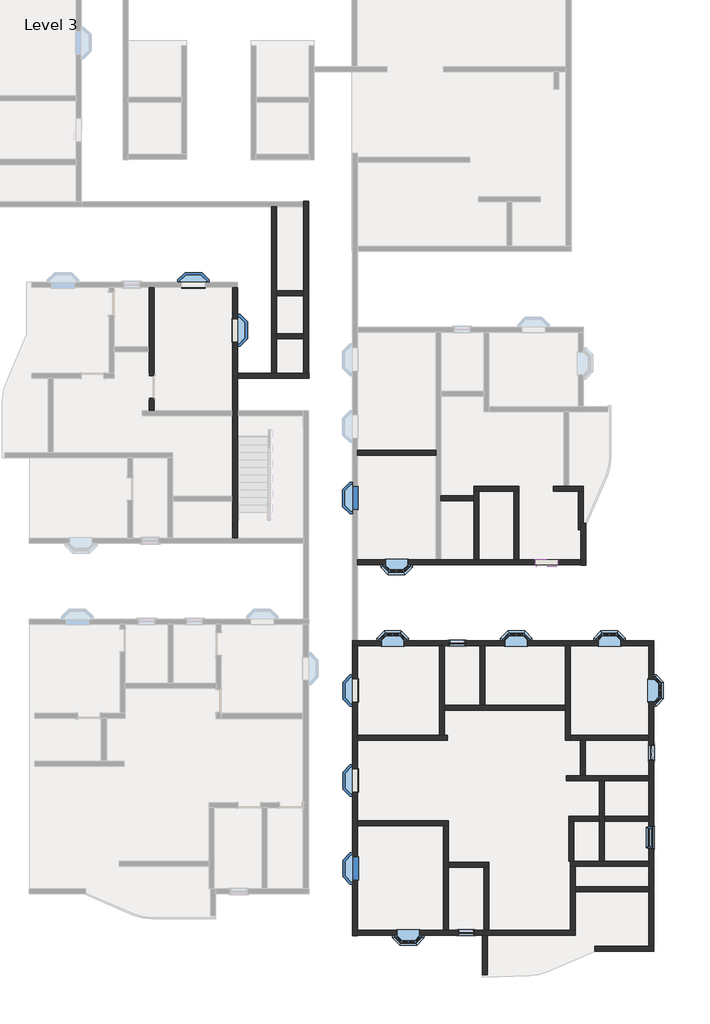
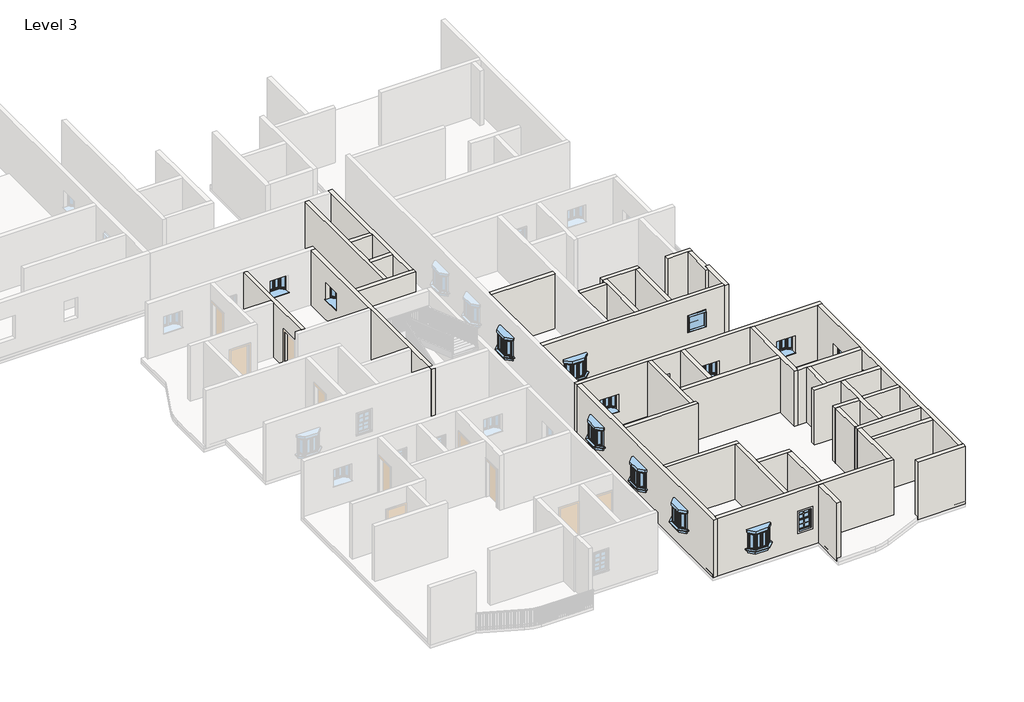
# One storey, part 2 of 14: 40 walls, 17 windows.
# Revit data of these elements (continued)
# Element 46 (IfcWindow, "910x910mm") (continued)
#   Materials on its faces: "Window Frame", "Glass"
# Element 47 (IfcWindow, "910x910mm")
#   Mark = "136"
#   Phase Created = New Construction
#   Materials on its faces: "Window Frame", "Glass"
# Element 48 (IfcWindow, "910x910mm")
#   Mark = "137"
#   Phase Created = New Construction
#   Materials on its faces: "Window Frame", "Glass"
# Element 49 (IfcWindow, "910x910mm")
#   Mark = "138"
#   Phase Created = New Construction
#   Materials on its faces: "Window Frame", "Glass"
# Element 50 (IfcWindow, "910x910mm")
#   Mark = "139"
#   Phase Created = New Construction
#   Materials on its faces: "Window Frame", "Glass"
# Element 51 (IfcWindow, "910x910mm")
#   Mark = "140"
#   Phase Created = New Construction
#   Materials on its faces: "Window Frame", "Glass"
# Element 52 (IfcWindow, "910x910mm")
#   Mark = "141"
#   Phase Created = New Construction
#   Materials on its faces: "Window Frame", "Glass"
# Element 53 (IfcWindow, "Window-Double-Hung : 26\" x 42\"")
#   Mark = "164"
#   Window Inset = 0' - 0"
#   Interior Wall Closure = 0' - 1 1/2"
#   Frame Extension = 0' - 1 1/4"
#   Exterior Wall Closure = 0' - 0 1/2"
#   Interior Trim Visibility = yes
#   Indicator Visibility = yes
#   Exterior Trim Visibility = yes
#   Phase Created = New Construction
#   Materials on its faces: "Wood - Stained", "Glass", "Clad - White"
# Element 54 (IfcWindow, "Window-Double-Hung : 26\" x 42\"")
#   Mark = "165"
#   Window Inset = 0' - 0"
#   Interior Wall Closure = 0' - 1 1/2"
#   Frame Extension = 0' - 1 1/4"
#   Exterior Wall Closure = 0' - 0 1/2"
#   Interior Trim Visibility = yes
#   Indicator Visibility = yes
#   Exterior Trim Visibility = yes
#   Phase Created = New Construction
#   Materials on its faces: "Wood - Stained", "Glass", "Clad - White"
# Element 55 (IfcWindow, "Window-Double-Hung : 26\" x 42\"")
#   Mark = "166"
#   Window Inset = 0' - 0"
#   Interior Wall Closure = 0' - 1 1/2"
#   Frame Extension = 0' - 1 1/4"
#   Exterior Wall Closure = 0' - 0 1/2"
#   Interior Trim Visibility = yes
#   Indicator Visibility = yes
#   Exterior Trim Visibility = yes
#   Phase Created = New Construction
#   Materials on its faces: "Wood - Stained", "Glass", "Clad - White"
# Element 56 (IfcWindow, "Windows_Sgl_w-Glazing_Bars : 910x910mm")
#   Mark = "154"
#   Phase Created = New Construction
#   Materials on its faces: "Window Frame", "Glass"
# Element 57 (IfcWindow, "Windows_Sgl_w-Glazing_Bars : 910x910mm")
#   Mark = "153"
#   Phase Created = New Construction
#   Materials on its faces: "Window Frame", "Glass"
# Materials
#   "Window Frame": colour RGB 249 249 249, transparency 0
#   "Glass": class "Glass", colour RGB 0 128 192, transparency 0.75, Description = "Soda Lime Glass", Cost = 0
#   "Wood - Stained": class "Wood", colour RGB 224 178 126, transparency 0, Cost = 0
#   "Clad - White": class "Wood", colour RGB 242 242 238, transparency 0, Cost = 0
#   "Default Wall": colour RGB 128 128 128, transparency 0, Cost = 0
#   "Door - Frame": colour RGB 118 70 51, transparency 0, Cost = 0
#   "Earth": class "Generic", colour RGB 97 75 62, transparency 0, Description = "Soil", Cost = 0
#   "Carpet (1)": class "Carpet", colour RGB 124 80 67, transparency 0, Description = "Interior finish", Cost = 0
#   "Acoustic Ceiling Tile 24 x 24": class "Generic", colour RGB 232 232 232, transparency 0, Description = "Acoustic Ceiling Tile 24 x 24", Cost = 0
